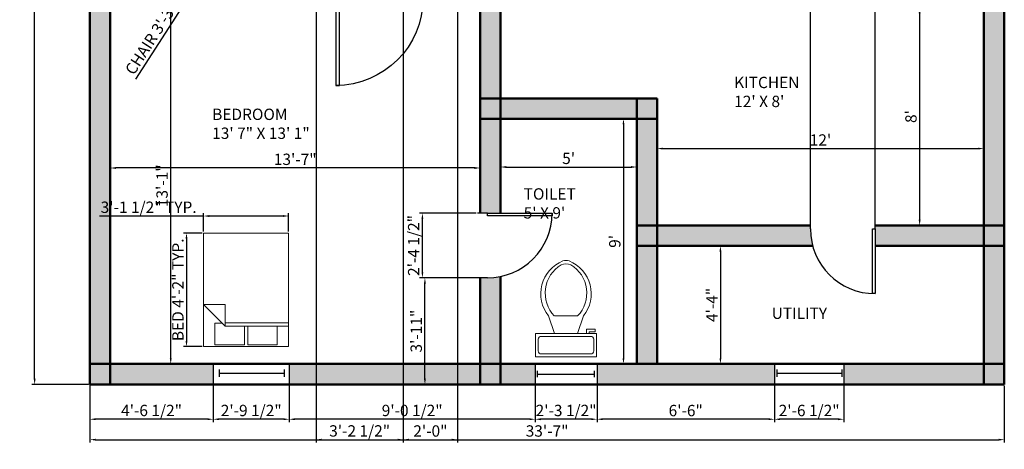
# Model space of a CAD drawing. Units: millimetres. Extents: x 3012 to 3478, y 929 to 1463.
# Tile 1 of 4: x 3012 to 3446, y 929 to 1118. Entities that reach past the tile are written whole.
import ezdxf

# ---------------------------------------------------------------- set-up
doc = ezdxf.new("R2010")
doc.units = ezdxf.units.MM
for name, color, linetype, lineweight in [('A-ANNO-DIMS', 50, 'Continuous', 18), ('A-AREA-IDEN', 170, 'Continuous', 25), ('A-FLOR-FIXT', 9, 'Continuous', 18), ('A-WALL-PATT', 252, 'Continuous', 13), ('doors', 130, 'Continuous', 25), ('furniture', 80, 'Continuous', 18), ('walls', 10, 'Continuous', 50), ('windows', 40, 'Continuous', 25)]:
    doc.layers.add(name, color=color, linetype=linetype, lineweight=lineweight)
doc.styles.get("Standard").update_dxf_attribs({"font": 'arial.ttf'})
doc.dimstyles.new('ISO-25', dxfattribs={"dimtxt": 5, "dimasz": 2.5, "dimexe": 1.25, "dimexo": 0.625, "dimtad": 1, "dimdec": 0, "dimlunit": 3, "dimtxsty": 'Standard', "dimcen": 2.5, "dimadec": 0, "dimazin": 0, "dimtfac": 1, "dimtdec": 0, "dimtmove": 0, "dimatfit": 3, "dimfxl": 1, "dimarcsym": 0})

# ---------------------------------------------------------------- blocks, each defined once
blk = doc.blocks.new('*U2')
for p, q in [((0, 0), (0, -6)), ((40, 0), (40, -6))]:
    blk.add_line(p, q)
blk.add_lwpolyline([(0, 0), (0, 40), (1.75, 40), (1.75, 0)], close=True)
blk.add_arc((0, 0), 40, 0, 90)
blk = doc.blocks.new('*U4')
for p, q in [((0, 4), (0, 0)), ((0, 2), (36, 2)), ((36, 4), (36, 0))]:
    blk.add_line(p, q)
blk = doc.blocks.new('*U5')
for p, q in [((0, 4), (0, 0)), ((0, 2), (36, 2)), ((36, 4), (36, 0))]:
    blk.add_line(p, q)
blk = doc.blocks.new('Bed - Queen')
for p, q in [((0, -80.00003), (0, 0)), ((0, 0), (59.99999, 0)), ((59.99999, 0), (59.99999, -80.00003)), ((7.99999, -1.2), (28.79998, -1.2)), ((7.99999, -14.4), (7.99999, -1.2)), ((28.79998, -1.2), (28.79998, -14.4)), ((31.19999, -1.2), (51.99999, -1.2)), ((31.19999, -14.4), (31.19999, -1.2)), ((51.99999, -1.2), (51.99999, -16.4)), ((0, -14.4), (44.8, -14.4)), ((44.8, -16.8), (0, -16.8)), ((59.99999, -29.6), (44.8, -14.4)), ((44.8, -14.4), (44.8, -29.6)), ((51.99999, -16.4), (46.79936, -16.4)), ((44.8, -29.6), (59.99999, -29.6)), ((59.99999, -80.00003), (0, -80.00003))]:
    blk.add_line(p, q)
blk = doc.blocks.new('Toilet - top')
for p, q in [((9.5, -6), (9.5, -2)), ((-10, -8.5), (-8, -8.5)), ((-10, -9.5), (-10, -8.5)), ((-7, -9.5), (-10, -9.5)), ((-8, -8.5), (-8, -8)), ((-7, -8), (-7, -9.5)), ((-4, -8), (-6, -14)), ((4, -8), (6, -14)), ((4, -14), (-4, -14))]:
    blk.add_line(p, q)
blk.add_lwpolyline([(10.5, -8), (10.5, 0), (-10.5, 0), (-10.5, -8)], close=True)
for points in [[(-9.5, -2), (-9.5, -6)], [(8.5, -1), (-8.5, -1)], [(-8.5, -7), (8.5, -7)]]:
    blk.add_lwpolyline(points)
for centre, radius, start, end in [((-8.62, -1.88), 0.884, 81.8699, 188.1301), ((8.62, -1.88), 0.884, 351.8699, 98.1301), ((-8.62, -6.12), 0.884, 171.8699, 278.1301), ((8.62, -6.12), 0.884, 261.8699, 8.1301), ((3.52, -21.58), 12.17, 141.4691, 247.9714), ((4.2, -21.82), 11.33, 136.3677, 238.9468), ((-3.52, -21.58), 12.17, 292.0284, 38.5307), ((-4.2, -21.82), 11.33, 301.053, 43.6321), ((0, -27.88), 4, 245.7318, 294.2682), ((0, -29), 4, 254.8605, 285.1395)]:
    blk.add_arc(centre, radius, start, end)
blk = doc.blocks.new('*D18')
at = {"layer": 'A-ANNO-DIMS', "color": 0, "lineweight": -2, "transparency": 16777216}
for p, q in [((3052.21, 1061.74), (3052.21, 1051.52)), ((3215.21, 1061.74), (3215.21, 1051.52)), ((3212.71, 1052.77), (3054.71, 1052.77))]:
    blk.add_line(p, q, dxfattribs=at)
at = {"layer": 'A-ANNO-DIMS', "color": 0, "transparency": 16777216}
for points in [[(3054.71, 1053.19), (3054.71, 1052.35), (3052.21, 1052.77)], [(3212.71, 1053.19), (3212.71, 1052.35), (3215.21, 1052.77)]]:
    blk.add_solid(points, dxfattribs=at)
at = {"layer": 'Defpoints', "color": 0, "transparency": 16777216}
for p in [(3052.21, 1062.37), (3215.21, 1062.37), (3052.21, 1052.77)]:
    blk.add_point(p, dxfattribs=at)
at = {"layer": 'A-ANNO-DIMS', "color": 0, "transparency": 16777216, "insert": (3133.71, 1055.95), "char_height": 5, "attachment_point": 5}
blk.add_mtext('13\'-7"', dxfattribs=at)
blk = doc.blocks.new('*D19')
at = {"layer": 'A-ANNO-DIMS', "color": 0, "lineweight": -2, "transparency": 16777216}
for p, q in [((3065.42, 1123.44), (3080.09, 1123.44)), ((3078.84, 968.94), (3078.84, 1120.94)), ((3065.42, 966.44), (3080.09, 966.44))]:
    blk.add_line(p, q, dxfattribs=at)
at = {"layer": 'A-ANNO-DIMS', "color": 0, "transparency": 16777216}
for points in [[(3078.43, 1120.94), (3079.26, 1120.94), (3078.84, 1123.44)], [(3078.43, 968.94), (3079.26, 968.94), (3078.84, 966.44)]]:
    blk.add_solid(points, dxfattribs=at)
at = {"layer": 'Defpoints', "color": 0, "transparency": 16777216}
for p in [(3064.8, 1123.44), (3078.84, 1123.44), (3064.8, 966.44)]:
    blk.add_point(p, dxfattribs=at)
at = {"layer": 'A-ANNO-DIMS', "color": 0, "transparency": 16777216, "insert": (3075.66, 1044.94), "char_height": 5, "attachment_point": 5, "rotation": 90}
blk.add_mtext('13\'-1"', dxfattribs=at)
blk = doc.blocks.new('*D20')
at = {"layer": 'A-ANNO-DIMS', "color": 0, "lineweight": -2, "transparency": 16777216}
for p, q in [((3277.29, 1074.44), (3279.62, 1074.44)), ((3278.37, 1071.94), (3278.37, 968.94)), ((3277.29, 966.44), (3279.62, 966.44))]:
    blk.add_line(p, q, dxfattribs=at)
at = {"layer": 'A-ANNO-DIMS', "color": 0, "transparency": 16777216}
for points in [[(3277.96, 1071.94), (3278.79, 1071.94), (3278.37, 1074.44)], [(3277.96, 968.94), (3278.79, 968.94), (3278.37, 966.44)]]:
    blk.add_solid(points, dxfattribs=at)
at = {"layer": 'Defpoints', "color": 0, "transparency": 16777216}
for p in [(3276.67, 1074.44), (3276.67, 966.44), (3278.37, 966.44)]:
    blk.add_point(p, dxfattribs=at)
at = {"layer": 'A-ANNO-DIMS', "color": 0, "transparency": 16777216, "insert": (3275.2, 1020.44), "char_height": 5, "attachment_point": 5, "rotation": 90}
blk.add_mtext("9'", dxfattribs=at)
blk = doc.blocks.new('*D21')
at = {"layer": 'A-ANNO-DIMS', "color": 0, "lineweight": -2, "transparency": 16777216}
for p, q in [((3224.21, 1053.83), (3224.21, 1054.45)), ((3226.71, 1053.2), (3281.71, 1053.2)), ((3284.21, 1053.83), (3284.21, 1054.45))]:
    blk.add_line(p, q, dxfattribs=at)
at = {"layer": 'A-ANNO-DIMS', "color": 0, "transparency": 16777216}
for points in [[(3226.71, 1053.62), (3226.71, 1052.78), (3224.21, 1053.2)], [(3281.71, 1053.62), (3281.71, 1052.78), (3284.21, 1053.2)]]:
    blk.add_solid(points, dxfattribs=at)
at = {"layer": 'Defpoints', "color": 0, "transparency": 16777216}
for p in [(3224.21, 1053.2), (3284.21, 1053.2), (3284.21, 1053.2)]:
    blk.add_point(p, dxfattribs=at)
at = {"layer": 'A-ANNO-DIMS', "color": 0, "transparency": 16777216, "insert": (3254.21, 1056.37), "char_height": 5, "attachment_point": 5}
blk.add_mtext("5'", dxfattribs=at)
blk = doc.blocks.new('*D22')
at = {"layer": 'A-ANNO-DIMS', "color": 0, "lineweight": -2, "transparency": 16777216}
for p, q in [((3322.37, 1018.44), (3319.85, 1018.44)), ((3321.1, 1015.94), (3321.1, 968.94)), ((3322.37, 966.44), (3319.85, 966.44))]:
    blk.add_line(p, q, dxfattribs=at)
at = {"layer": 'A-ANNO-DIMS', "color": 0, "transparency": 16777216}
for points in [[(3320.68, 1015.94), (3321.51, 1015.94), (3321.1, 1018.44)], [(3320.68, 968.94), (3321.51, 968.94), (3321.1, 966.44)]]:
    blk.add_solid(points, dxfattribs=at)
at = {"layer": 'Defpoints', "color": 0, "transparency": 16777216}
for p in [(3322.99, 1018.44), (3321.1, 966.44), (3322.99, 966.44)]:
    blk.add_point(p, dxfattribs=at)
at = {"layer": 'A-ANNO-DIMS', "color": 0, "transparency": 16777216, "insert": (3317.97, 992.44), "char_height": 5, "attachment_point": 5, "rotation": 90}
blk.add_mtext('4\'-4"', dxfattribs=at)
blk = doc.blocks.new('*D23')
at = {"layer": 'A-ANNO-DIMS', "color": 0, "lineweight": -2, "transparency": 16777216}
for p, q in [((3408.9, 1120.94), (3408.9, 1029.94)), ((3409.52, 1123.44), (3410.15, 1123.44)), ((3409.52, 1027.44), (3410.15, 1027.44))]:
    blk.add_line(p, q, dxfattribs=at)
at = {"layer": 'A-ANNO-DIMS', "color": 0, "transparency": 16777216}
for points in [[(3408.48, 1120.94), (3409.31, 1120.94), (3408.9, 1123.44)], [(3408.48, 1029.94), (3409.31, 1029.94), (3408.9, 1027.44)]]:
    blk.add_solid(points, dxfattribs=at)
at = {"layer": 'Defpoints', "color": 0, "transparency": 16777216}
for p in [(3408.9, 1123.44), (3408.9, 1027.44), (3408.9, 1027.44)]:
    blk.add_point(p, dxfattribs=at)
at = {"layer": 'A-ANNO-DIMS', "color": 0, "transparency": 16777216, "insert": (3405.72, 1075.44), "char_height": 5, "attachment_point": 5, "rotation": 90}
blk.add_mtext("8'", dxfattribs=at)
blk = doc.blocks.new('*D24')
at = {"layer": 'A-ANNO-DIMS', "color": 0, "lineweight": -2, "transparency": 16777216}
for p, q in [((3293.21, 1055.32), (3293.21, 1062.57)), ((3295.71, 1061.32), (3434.71, 1061.32)), ((3437.21, 1055.32), (3437.21, 1062.57))]:
    blk.add_line(p, q, dxfattribs=at)
at = {"layer": 'A-ANNO-DIMS', "color": 0, "transparency": 16777216}
for points in [[(3295.71, 1061.74), (3295.71, 1060.91), (3293.21, 1061.32)], [(3434.71, 1061.74), (3434.71, 1060.91), (3437.21, 1061.32)]]:
    blk.add_solid(points, dxfattribs=at)
at = {"layer": 'Defpoints', "color": 0, "transparency": 16777216}
for p in [(3437.21, 1061.32), (3293.21, 1054.7), (3437.21, 1054.7)]:
    blk.add_point(p, dxfattribs=at)
at = {"layer": 'A-ANNO-DIMS', "color": 0, "transparency": 16777216, "insert": (3365.21, 1064.46), "char_height": 5, "attachment_point": 5}
blk.add_mtext("12'", dxfattribs=at)
blk = doc.blocks.new('*D30')
at = {"layer": 'A-ANNO-DIMS', "color": 0, "lineweight": -2, "transparency": 16777216}
for p, q in [((3092.67, 1024.12), (3084.54, 1024.12)), ((3085.79, 1021.62), (3085.79, 976.61)), ((3092.67, 974.11), (3084.54, 974.11))]:
    blk.add_line(p, q, dxfattribs=at)
at = {"layer": 'A-ANNO-DIMS', "color": 0, "transparency": 16777216}
for points in [[(3085.38, 1021.62), (3086.21, 1021.62), (3085.79, 1024.12)], [(3085.38, 976.61), (3086.21, 976.61), (3085.79, 974.11)]]:
    blk.add_solid(points, dxfattribs=at)
at = {"layer": 'Defpoints', "color": 0, "transparency": 16777216}
for p in [(3093.3, 1024.12), (3085.79, 974.11), (3093.3, 974.11)]:
    blk.add_point(p, dxfattribs=at)
at = {"layer": 'A-ANNO-DIMS', "color": 0, "transparency": 16777216, "insert": (3082.66, 999.11), "char_height": 5, "attachment_point": 5, "rotation": 90}
blk.add_mtext('BED 4\'-2" TYP.', dxfattribs=at)
blk = doc.blocks.new('*D31')
at = {"layer": 'A-ANNO-DIMS', "color": 0, "lineweight": -2, "transparency": 16777216}
for p, q in [((3093.3, 1024.74), (3093.3, 1032.87)), ((3130.81, 1024.74), (3130.81, 1032.87)), ((3093.3, 1031.62), (3047.42, 1031.62)), ((3128.31, 1031.62), (3095.8, 1031.62))]:
    blk.add_line(p, q, dxfattribs=at)
at = {"layer": 'A-ANNO-DIMS', "color": 0, "transparency": 16777216}
for points in [[(3095.8, 1032.04), (3095.8, 1031.2), (3093.3, 1031.62)], [(3128.31, 1032.04), (3128.31, 1031.2), (3130.81, 1031.62)]]:
    blk.add_solid(points, dxfattribs=at)
at = {"layer": 'Defpoints', "color": 0, "transparency": 16777216}
for p in [(3093.3, 1031.62), (3093.3, 1024.12), (3130.81, 1024.12)]:
    blk.add_point(p, dxfattribs=at)
at = {"layer": 'A-ANNO-DIMS', "color": 0, "transparency": 16777216, "insert": (3069.11, 1034.83), "char_height": 5, "attachment_point": 5}
blk.add_mtext('3\'-1 1/2" TYP.', dxfattribs=at)
blk = doc.blocks.new('*D40')
at = {"layer": 'A-ANNO-DIMS', "color": 0, "lineweight": -2, "transparency": 16777216}
for p, q in [((3108.55, 1171.79), (3114.04, 1168.25)), ((3111.63, 1166.83), (3093, 1137.95)), ((3087.21, 1138.72), (3092.7, 1135.18)), ((3091.65, 1135.85), (3063.29, 1091.9))]:
    blk.add_line(p, q, dxfattribs=at)
at = {"layer": 'A-ANNO-DIMS', "color": 0, "transparency": 16777216}
for points in [[(3111.28, 1167.05), (3111.98, 1166.6), (3112.99, 1168.93)], [(3092.65, 1138.18), (3093.35, 1137.73), (3091.65, 1135.85)]]:
    blk.add_solid(points, dxfattribs=at)
at = {"layer": 'Defpoints', "color": 0, "transparency": 16777216}
for p in [(3108.03, 1172.13), (3086.69, 1139.06), (3091.65, 1135.85)]:
    blk.add_point(p, dxfattribs=at)
at = {"layer": 'A-ANNO-DIMS', "color": 0, "transparency": 16777216, "insert": (3074.09, 1114.57), "char_height": 5, "attachment_point": 5, "rotation": 57.1659}
blk.add_mtext('CHAIR 3\'-3 1/2"', dxfattribs=at)
blk = doc.blocks.new('*D42')
at = {"layer": 'A-ANNO-DIMS', "color": 0, "lineweight": -2, "transparency": 16777216}
for p, q in [((3042.59, 1414.44), (3017.61, 1414.44)), ((3018.86, 959.94), (3018.86, 1411.94)), ((3042.59, 957.44), (3017.61, 957.44))]:
    blk.add_line(p, q, dxfattribs=at)
at = {"layer": 'A-ANNO-DIMS', "color": 0, "transparency": 16777216}
for points in [[(3018.45, 1411.94), (3019.28, 1411.94), (3018.86, 1414.44)], [(3018.45, 959.94), (3019.28, 959.94), (3018.86, 957.44)]]:
    blk.add_solid(points, dxfattribs=at)
at = {"layer": 'Defpoints', "color": 0, "transparency": 16777216}
for p in [(3018.86, 1414.44), (3043.21, 1414.44), (3043.21, 957.44)]:
    blk.add_point(p, dxfattribs=at)
at = {"layer": 'A-ANNO-DIMS', "color": 0, "transparency": 16777216, "insert": (3015.68, 1185.94), "char_height": 5, "attachment_point": 5, "rotation": 90}
blk.add_mtext('38\'-1"', dxfattribs=at)
blk = doc.blocks.new('*D49')
at = {"layer": 'A-ANNO-DIMS', "color": 0, "lineweight": -2, "transparency": 16777216}
for p, q in [((3043.21, 965.82), (3043.21, 940.84)), ((3097.57, 965.82), (3097.57, 940.84)), ((3095.07, 942.09), (3045.71, 942.09))]:
    blk.add_line(p, q, dxfattribs=at)
at = {"layer": 'A-ANNO-DIMS', "color": 0, "transparency": 16777216}
for points in [[(3045.71, 942.51), (3045.71, 941.68), (3043.21, 942.09)], [(3095.07, 942.51), (3095.07, 941.68), (3097.57, 942.09)]]:
    blk.add_solid(points, dxfattribs=at)
at = {"layer": 'Defpoints', "color": 0, "transparency": 16777216}
for p in [(3043.21, 966.44), (3097.57, 966.44), (3043.21, 942.09)]:
    blk.add_point(p, dxfattribs=at)
at = {"layer": 'A-ANNO-DIMS', "color": 0, "transparency": 16777216, "insert": (3070.39, 945.3), "char_height": 5, "attachment_point": 5}
blk.add_mtext('4\'-6 1/2"', dxfattribs=at)
blk = doc.blocks.new('*D50')
at = {"layer": 'A-ANNO-DIMS', "color": 0, "lineweight": -2, "transparency": 16777216}
for p, q in [((3097.57, 965.82), (3097.57, 940.84)), ((3131.05, 965.82), (3131.05, 940.84)), ((3128.55, 942.09), (3100.07, 942.09))]:
    blk.add_line(p, q, dxfattribs=at)
at = {"layer": 'A-ANNO-DIMS', "color": 0, "transparency": 16777216}
for points in [[(3100.07, 942.51), (3100.07, 941.68), (3097.57, 942.09)], [(3128.55, 942.51), (3128.55, 941.68), (3131.05, 942.09)]]:
    blk.add_solid(points, dxfattribs=at)
at = {"layer": 'Defpoints', "color": 0, "transparency": 16777216}
for p in [(3097.57, 966.44), (3131.05, 966.44), (3097.57, 942.09)]:
    blk.add_point(p, dxfattribs=at)
at = {"layer": 'A-ANNO-DIMS', "color": 0, "transparency": 16777216, "insert": (3114.31, 945.3), "char_height": 5, "attachment_point": 5}
blk.add_mtext('2\'-9 1/2"', dxfattribs=at)
blk = doc.blocks.new('*D51')
at = {"layer": 'A-ANNO-DIMS', "color": 0, "lineweight": -2, "transparency": 16777216}
for p, q in [((3131.05, 965.82), (3131.05, 940.84)), ((3239.46, 965.82), (3239.46, 940.84)), ((3236.96, 942.09), (3133.55, 942.09))]:
    blk.add_line(p, q, dxfattribs=at)
at = {"layer": 'A-ANNO-DIMS', "color": 0, "transparency": 16777216}
for points in [[(3133.55, 942.51), (3133.55, 941.68), (3131.05, 942.09)], [(3236.96, 942.51), (3236.96, 941.68), (3239.46, 942.09)]]:
    blk.add_solid(points, dxfattribs=at)
at = {"layer": 'Defpoints', "color": 0, "transparency": 16777216}
for p in [(3131.05, 966.44), (3239.46, 966.44), (3131.05, 942.09)]:
    blk.add_point(p, dxfattribs=at)
at = {"layer": 'A-ANNO-DIMS', "color": 0, "transparency": 16777216, "insert": (3185.25, 945.3), "char_height": 5, "attachment_point": 5}
blk.add_mtext('9\'-0 1/2"', dxfattribs=at)
blk = doc.blocks.new('*D52')
at = {"layer": 'A-ANNO-DIMS', "color": 0, "lineweight": -2, "transparency": 16777216}
for p, q in [((3239.46, 965.82), (3239.46, 940.84)), ((3266.71, 965.82), (3266.71, 940.84)), ((3264.21, 942.09), (3241.96, 942.09))]:
    blk.add_line(p, q, dxfattribs=at)
at = {"layer": 'A-ANNO-DIMS', "color": 0, "transparency": 16777216}
for points in [[(3241.96, 942.51), (3241.96, 941.68), (3239.46, 942.09)], [(3264.21, 942.51), (3264.21, 941.68), (3266.71, 942.09)]]:
    blk.add_solid(points, dxfattribs=at)
at = {"layer": 'Defpoints', "color": 0, "transparency": 16777216}
for p in [(3239.46, 966.44), (3266.71, 966.44), (3239.46, 942.09)]:
    blk.add_point(p, dxfattribs=at)
at = {"layer": 'A-ANNO-DIMS', "color": 0, "transparency": 16777216, "insert": (3253.08, 945.3), "char_height": 5, "attachment_point": 5}
blk.add_mtext('2\'-3 1/2"', dxfattribs=at)
blk = doc.blocks.new('*D53')
at = {"layer": 'A-ANNO-DIMS', "color": 0, "lineweight": -2, "transparency": 16777216}
for p, q in [((3266.71, 965.82), (3266.71, 940.84)), ((3344.91, 965.82), (3344.91, 940.84)), ((3342.41, 942.09), (3269.21, 942.09))]:
    blk.add_line(p, q, dxfattribs=at)
at = {"layer": 'A-ANNO-DIMS', "color": 0, "transparency": 16777216}
for points in [[(3269.21, 942.51), (3269.21, 941.68), (3266.71, 942.09)], [(3342.41, 942.51), (3342.41, 941.68), (3344.91, 942.09)]]:
    blk.add_solid(points, dxfattribs=at)
at = {"layer": 'Defpoints', "color": 0, "transparency": 16777216}
for p in [(3266.71, 966.44), (3344.91, 966.44), (3266.71, 942.09)]:
    blk.add_point(p, dxfattribs=at)
at = {"layer": 'A-ANNO-DIMS', "color": 0, "transparency": 16777216, "insert": (3305.81, 945.27), "char_height": 5, "attachment_point": 5}
blk.add_mtext('6\'-6"', dxfattribs=at)
blk = doc.blocks.new('*D54')
at = {"layer": 'A-ANNO-DIMS', "color": 0, "lineweight": -2, "transparency": 16777216}
for p, q in [((3344.91, 965.82), (3344.91, 940.84)), ((3375.49, 965.82), (3375.49, 940.84)), ((3372.99, 942.09), (3347.41, 942.09))]:
    blk.add_line(p, q, dxfattribs=at)
at = {"layer": 'A-ANNO-DIMS', "color": 0, "transparency": 16777216}
for points in [[(3347.41, 942.51), (3347.41, 941.68), (3344.91, 942.09)], [(3372.99, 942.51), (3372.99, 941.68), (3375.49, 942.09)]]:
    blk.add_solid(points, dxfattribs=at)
at = {"layer": 'Defpoints', "color": 0, "transparency": 16777216}
for p in [(3344.91, 966.44), (3375.49, 966.44), (3344.91, 942.09)]:
    blk.add_point(p, dxfattribs=at)
at = {"layer": 'A-ANNO-DIMS', "color": 0, "transparency": 16777216, "insert": (3360.2, 945.3), "char_height": 5, "attachment_point": 5}
blk.add_mtext('2\'-6 1/2"', dxfattribs=at)
blk = doc.blocks.new('*D57')
at = {"layer": 'A-ANNO-DIMS', "color": 0, "lineweight": -2, "transparency": 16777216}
for p, q in [((3142.87, 1263.82), (3142.87, 931.84)), ((3181.32, 1263.82), (3181.32, 931.84)), ((3145.37, 933.09), (3178.82, 933.09))]:
    blk.add_line(p, q, dxfattribs=at)
at = {"layer": 'A-ANNO-DIMS', "color": 0, "transparency": 16777216}
for points in [[(3145.37, 933.51), (3145.37, 932.68), (3142.87, 933.09)], [(3178.82, 933.51), (3178.82, 932.68), (3181.32, 933.09)]]:
    blk.add_solid(points, dxfattribs=at)
at = {"layer": 'Defpoints', "color": 0, "transparency": 16777216}
for p in [(3142.87, 1264.44), (3181.32, 1264.44), (3181.32, 933.09)]:
    blk.add_point(p, dxfattribs=at)
at = {"layer": 'A-ANNO-DIMS', "color": 0, "transparency": 16777216, "insert": (3162.1, 936.3), "char_height": 5, "attachment_point": 5}
blk.add_mtext('3\'-2 1/2"', dxfattribs=at)
blk = doc.blocks.new('*D58')
at = {"layer": 'A-ANNO-DIMS', "color": 0, "lineweight": -2, "transparency": 16777216}
for p, q in [((3181.32, 1263.82), (3181.32, 931.84)), ((3205.21, 1263.82), (3205.21, 931.84)), ((3183.82, 933.09), (3202.71, 933.09))]:
    blk.add_line(p, q, dxfattribs=at)
at = {"layer": 'A-ANNO-DIMS', "color": 0, "transparency": 16777216}
for points in [[(3183.82, 933.51), (3183.82, 932.68), (3181.32, 933.09)], [(3202.71, 933.51), (3202.71, 932.68), (3205.21, 933.09)]]:
    blk.add_solid(points, dxfattribs=at)
at = {"layer": 'Defpoints', "color": 0, "transparency": 16777216}
for p in [(3181.32, 1264.44), (3205.21, 1264.44), (3205.21, 933.09)]:
    blk.add_point(p, dxfattribs=at)
at = {"layer": 'A-ANNO-DIMS', "color": 0, "transparency": 16777216, "insert": (3193.27, 936.27), "char_height": 5, "attachment_point": 5}
blk.add_mtext('2\'-0"', dxfattribs=at)
blk = doc.blocks.new('*D63')
at = {"layer": 'A-ANNO-DIMS', "color": 0, "lineweight": -2, "transparency": 16777216}
for p, q in [((3213.49, 1032.91), (3188.51, 1032.91)), ((3189.76, 1006.87), (3189.76, 1030.41)), ((3213.49, 1004.37), (3188.51, 1004.37))]:
    blk.add_line(p, q, dxfattribs=at)
at = {"layer": 'A-ANNO-DIMS', "color": 0, "transparency": 16777216}
for points in [[(3189.34, 1030.41), (3190.18, 1030.41), (3189.76, 1032.91)], [(3189.34, 1006.87), (3190.18, 1006.87), (3189.76, 1004.37)]]:
    blk.add_solid(points, dxfattribs=at)
at = {"layer": 'Defpoints', "color": 0, "transparency": 16777216}
for p in [(3189.76, 1032.91), (3214.11, 1032.91), (3214.11, 1004.37)]:
    blk.add_point(p, dxfattribs=at)
at = {"layer": 'A-ANNO-DIMS', "color": 0, "transparency": 16777216, "insert": (3186.55, 1018.64), "char_height": 5, "attachment_point": 5, "rotation": 90}
blk.add_mtext('2\'-4 1/2"', dxfattribs=at)
blk = doc.blocks.new('*D64')
at = {"layer": 'A-ANNO-DIMS', "color": 0, "lineweight": -2, "transparency": 16777216}
for p, q in [((3214.59, 1004.37), (3189.61, 1004.37)), ((3190.86, 959.94), (3190.86, 1001.87)), ((3214.59, 957.44), (3189.61, 957.44))]:
    blk.add_line(p, q, dxfattribs=at)
at = {"layer": 'A-ANNO-DIMS', "color": 0, "transparency": 16777216}
for points in [[(3190.45, 1001.87), (3191.28, 1001.87), (3190.86, 1004.37)], [(3190.45, 959.94), (3191.28, 959.94), (3190.86, 957.44)]]:
    blk.add_solid(points, dxfattribs=at)
at = {"layer": 'Defpoints', "color": 0, "transparency": 16777216}
for p in [(3190.86, 1004.37), (3215.21, 1004.37), (3215.21, 957.44)]:
    blk.add_point(p, dxfattribs=at)
at = {"layer": 'A-ANNO-DIMS', "color": 0, "transparency": 16777216, "insert": (3187.68, 980.91), "char_height": 5, "attachment_point": 5, "rotation": 90}
blk.add_mtext('3\'-11"', dxfattribs=at)
blk = doc.blocks.new('*D65')
at = {"layer": 'A-ANNO-DIMS', "color": 0, "lineweight": -2, "transparency": 16777216}
for p, q in [((3360.77, 1028.07), (3360.77, 1440.04)), ((3363.27, 1438.79), (3386.8, 1438.79)), ((3389.3, 1028.07), (3389.3, 1440.04))]:
    blk.add_line(p, q, dxfattribs=at)
at = {"layer": 'A-ANNO-DIMS', "color": 0, "transparency": 16777216}
for points in [[(3363.27, 1439.21), (3363.27, 1438.38), (3360.77, 1438.79)], [(3386.8, 1439.21), (3386.8, 1438.38), (3389.3, 1438.79)]]:
    blk.add_solid(points, dxfattribs=at)
at = {"layer": 'Defpoints', "color": 0, "transparency": 16777216}
for p in [(3389.3, 1438.79), (3360.77, 1027.44), (3389.3, 1027.44)]:
    blk.add_point(p, dxfattribs=at)
at = {"layer": 'A-ANNO-DIMS', "color": 0, "transparency": 16777216, "insert": (3375.03, 1442), "char_height": 5, "attachment_point": 5}
blk.add_mtext('2\'-4 1/2"', dxfattribs=at)
blk = doc.blocks.new('*D66')
at = {"layer": 'A-ANNO-DIMS', "color": 0, "lineweight": -2, "transparency": 16777216}
for p, q in [((3389.3, 1028.07), (3389.3, 1440.04)), ((3391.8, 1438.79), (3443.71, 1438.79)), ((3446.21, 1028.07), (3446.21, 1440.04))]:
    blk.add_line(p, q, dxfattribs=at)
at = {"layer": 'A-ANNO-DIMS', "color": 0, "transparency": 16777216}
for points in [[(3391.8, 1439.21), (3391.8, 1438.38), (3389.3, 1438.79)], [(3443.71, 1439.21), (3443.71, 1438.38), (3446.21, 1438.79)]]:
    blk.add_solid(points, dxfattribs=at)
at = {"layer": 'Defpoints', "color": 0, "transparency": 16777216}
for p in [(3446.21, 1438.79), (3389.3, 1027.44), (3446.21, 1027.44)]:
    blk.add_point(p, dxfattribs=at)
at = {"layer": 'A-ANNO-DIMS', "color": 0, "transparency": 16777216, "insert": (3417.76, 1441.97), "char_height": 5, "attachment_point": 5}
blk.add_mtext('4\'-9"', dxfattribs=at)
blk = doc.blocks.new('*D74')
at = {"layer": 'A-ANNO-DIMS', "color": 0, "lineweight": -2, "transparency": 16777216}
for p, q in [((3043.21, 956.82), (3043.21, 931.84)), ((3446.21, 956.82), (3446.21, 931.84)), ((3045.71, 933.09), (3443.71, 933.09))]:
    blk.add_line(p, q, dxfattribs=at)
at = {"layer": 'A-ANNO-DIMS', "color": 0, "transparency": 16777216}
for points in [[(3045.71, 933.51), (3045.71, 932.68), (3043.21, 933.09)], [(3443.71, 933.51), (3443.71, 932.68), (3446.21, 933.09)]]:
    blk.add_solid(points, dxfattribs=at)
at = {"layer": 'Defpoints', "color": 0, "transparency": 16777216}
for p in [(3043.21, 957.44), (3446.21, 957.44), (3446.21, 933.09)]:
    blk.add_point(p, dxfattribs=at)
at = {"layer": 'A-ANNO-DIMS', "color": 0, "transparency": 16777216, "insert": (3244.71, 936.27), "char_height": 5, "attachment_point": 5}
blk.add_mtext('33\'-7"', dxfattribs=at)

msp = doc.modelspace()

# ---------------------------------------------------------------- hatches: boundary and pattern name
at = {"layer": 'A-WALL-PATT'}
h = msp.add_hatch(color=256, dxfattribs=at)
h.dxf.hatch_style = 1
h.paths.add_polyline_path([(3052.21, 1405.44), (3043.21, 1405.44), (3043.21, 1273.44), (3052.21, 1273.44)])
h.paths.add_polyline_path([(3052.21, 1273.44), (3043.21, 1273.44), (3043.21, 1264.44), (3052.21, 1264.44)])
h.paths.add_polyline_path([(3052.21, 1264.44), (3043.21, 1264.44), (3043.21, 1132.44), (3052.21, 1132.44)])
h.paths.add_polyline_path([(3116.21, 1273.44), (3052.21, 1273.44), (3052.21, 1264.44), (3116.21, 1264.44)])
h.paths.add_polyline_path([(3125.21, 1273.44), (3116.21, 1273.44), (3116.21, 1264.44), (3125.21, 1264.44)])
h.paths.add_polyline_path([(3143.26, 1273.44), (3125.21, 1273.44), (3125.21, 1264.44), (3142.87, 1264.44), (3142.87, 1268, -0.035543)])
h.paths.add_polyline_path([(3052.21, 1414.44), (3043.21, 1414.44), (3043.21, 1405.44), (3052.21, 1405.44)])
h.paths.add_polyline_path([(3096.89, 1414.44), (3052.21, 1414.44), (3052.21, 1405.44), (3096.89, 1405.44)])
h.paths.add_polyline_path([(3196.21, 1414.44), (3129.12, 1414.44), (3129.12, 1405.44), (3196.21, 1405.44)])
h.paths.add_polyline_path([(3205.21, 1414.44), (3196.21, 1414.44), (3196.21, 1405.44), (3205.21, 1405.44)])
h.paths.add_polyline_path([(3205.21, 1405.44), (3196.21, 1405.44), (3196.21, 1321.44), (3205.21, 1321.44)])
h.paths.add_polyline_path([(3205.21, 1321.44), (3196.21, 1321.44), (3196.21, 1312.44), (3205.21, 1312.44)])
h.paths.add_polyline_path([(3205.21, 1312.44), (3196.21, 1312.44), (3196.21, 1273.44), (3205.21, 1273.44)])
h.paths.add_polyline_path([(3284.21, 1321.44), (3205.21, 1321.44), (3205.21, 1312.44), (3284.21, 1312.44)])
h.paths.add_polyline_path([(3205.21, 1273.44), (3196.21, 1273.44), (3196.21, 1264.44), (3205.21, 1264.44)])
h.paths.add_polyline_path([(3196.21, 1273.44), (3181.32, 1273.44), (3181.32, 1268), (3181.32, 1264.44), (3196.21, 1264.44)])
h.paths.add_polyline_path([(3293.21, 1405.44), (3284.21, 1405.44), (3284.21, 1321.44), (3293.21, 1321.44)])
h.paths.add_polyline_path([(3293.21, 1414.44), (3284.21, 1414.44), (3284.21, 1405.44), (3293.21, 1405.44)])
h.paths.add_polyline_path([(3284.21, 1414.44), (3249.55, 1414.44), (3249.55, 1405.44), (3284.21, 1405.44)])
h.paths.add_polyline_path([(3221.79, 1414.44), (3205.21, 1414.44), (3205.21, 1405.44), (3221.79, 1405.44)])
h.paths.add_polyline_path([(3339.87, 1414.44), (3293.21, 1414.44), (3293.21, 1405.44), (3339.87, 1405.44)])
h.paths.add_polyline_path([(3437.21, 1414.44), (3373.17, 1414.44), (3373.17, 1405.44), (3437.21, 1405.44)])
h.paths.add_polyline_path([(3446.21, 1414.44), (3437.21, 1414.44), (3437.21, 1405.44), (3446.21, 1405.44)])
h.paths.add_polyline_path([(3446.21, 1405.44), (3437.21, 1405.44), (3437.21, 1273.44), (3446.21, 1273.44)])
h.paths.add_polyline_path([(3437.21, 1273.44), (3293.21, 1273.44), (3293.21, 1264.44), (3437.21, 1264.44)])
h.paths.add_polyline_path([(3446.21, 1273.44), (3437.21, 1273.44), (3437.21, 1264.44), (3446.21, 1264.44)])
h.paths.add_polyline_path([(3446.21, 1264.44), (3437.21, 1264.44), (3437.21, 1249.83), (3445.52, 1249.83), (3446.21, 1249.83)])
h.paths.add_polyline_path([(3293.21, 1264.44), (3284.21, 1264.44), (3284.21, 1132.44), (3293.21, 1132.44)])
h.paths.add_polyline_path([(3293.21, 1273.44), (3284.21, 1273.44), (3284.21, 1264.44), (3293.21, 1264.44)])
h.paths.add_polyline_path([(3293.21, 1277.22), (3287.47, 1277.22), (3284.21, 1277.22), (3284.21, 1273.44), (3293.21, 1273.44)])
h.paths.add_polyline_path([(3125.21, 1213.86), (3116.21, 1213.86), (3116.21, 1184.42), (3125.21, 1184.42)])
h.paths.add_polyline_path([(3125.21, 1264.44), (3116.21, 1264.44), (3116.21, 1245.36), (3125.21, 1245.36)])
h.paths.add_polyline_path([(3125.21, 1151.51), (3116.21, 1151.51), (3116.21, 1132.44), (3125.21, 1132.44)])
h.paths.add_polyline_path([(3125.21, 1132.44), (3116.21, 1132.44), (3116.21, 1123.44), (3125.21, 1123.44)])
h.paths.add_polyline_path([(3151.56, 1127.56), (3151.56, 1132.44), (3125.21, 1132.44), (3125.21, 1123.44), (3151.56, 1123.44)])
h.paths.add_polyline_path([(3116.21, 1132.44), (3052.21, 1132.44), (3052.21, 1123.44), (3116.21, 1123.44)])
h.paths.add_polyline_path([(3052.21, 1132.44), (3043.21, 1132.44), (3043.21, 1123.44), (3052.21, 1123.44)])
h.paths.add_polyline_path([(3052.21, 1123.44), (3043.21, 1123.44), (3043.21, 966.44), (3052.21, 966.44)])
h.paths.add_polyline_path([(3097.57, 966.44), (3052.21, 966.44), (3052.21, 957.44), (3097.57, 957.44)])
h.paths.add_polyline_path([(3052.21, 966.44), (3043.21, 966.44), (3043.21, 957.44), (3052.21, 957.44)])
h.paths.add_polyline_path([(3215.21, 966.44), (3131.05, 966.44), (3131.05, 957.44), (3215.21, 957.44)])
h.paths.add_polyline_path([(3224.21, 966.44), (3215.21, 966.44), (3215.21, 957.44), (3224.21, 957.44)])
h.paths.add_polyline_path([(3224.21, 1004.97, -0.051409), (3218.39, 1004.37), (3215.21, 1004.37), (3215.21, 966.44), (3224.21, 966.44)])
h.paths.add_polyline_path([(3239.46, 966.44), (3224.21, 966.44), (3224.21, 957.44), (3239.46, 957.44)])
h.paths.add_polyline_path([(3344.91, 966.44), (3266.71, 966.44), (3266.71, 957.44), (3344.91, 957.44)])
h.paths.add_polyline_path([(3293.21, 1018.44), (3284.21, 1018.44), (3284.21, 966.44), (3293.21, 966.44)])
h.paths.add_polyline_path([(3293.21, 1027.44), (3284.21, 1027.44), (3284.21, 1018.44), (3293.21, 1018.44)])
h.paths.add_polyline_path([(3293.21, 1074.44), (3284.21, 1074.44), (3284.21, 1027.44), (3293.21, 1027.44)])
h.paths.add_polyline_path([(3224.21, 1074.44), (3215.21, 1074.44), (3215.21, 1032.91), (3218.39, 1032.91), (3224.21, 1032.91)])
h.paths.add_polyline_path([(3224.21, 1123.44), (3215.21, 1123.44), (3215.21, 1083.44), (3224.21, 1083.44)])
h.paths.add_polyline_path([(3224.21, 1083.44), (3215.21, 1083.44), (3215.21, 1074.44), (3224.21, 1074.44)])
h.paths.add_polyline_path([(3284.21, 1083.44), (3224.21, 1083.44), (3224.21, 1074.44), (3284.21, 1074.44)])
h.paths.add_polyline_path([(3293.21, 1083.44), (3284.21, 1083.44), (3284.21, 1074.44), (3293.21, 1074.44)])
h.paths.add_polyline_path([(3215.21, 1132.44), (3190.01, 1132.44), (3190.01, 1127.56, -0.026825), (3189.79, 1123.44), (3215.21, 1123.44)])
h.paths.add_polyline_path([(3224.21, 1132.44), (3215.21, 1132.44), (3215.21, 1123.44), (3224.21, 1123.44)])
h.paths.add_polyline_path([(3437.21, 1132.44), (3293.21, 1132.44), (3293.21, 1123.44), (3437.21, 1123.44)])
h.paths.add_polyline_path([(3293.21, 1132.44), (3284.21, 1132.44), (3284.21, 1123.44), (3293.21, 1123.44)])
h.paths.add_polyline_path([(3446.21, 1132.44), (3437.21, 1132.44), (3437.21, 1123.44), (3446.21, 1123.44)])
h.paths.add_polyline_path([(3446.21, 1123.44), (3437.21, 1123.44), (3437.21, 1027.44), (3446.21, 1027.44)])
h.paths.add_polyline_path([(3446.21, 1221.29), (3445.52, 1221.29, -0.074007), (3437.21, 1222.53), (3437.21, 1132.44), (3446.21, 1132.44)])
h.paths.add_polyline_path([(3446.21, 1018.44), (3437.21, 1018.44), (3437.21, 966.44), (3446.21, 966.44)])
h.paths.add_polyline_path([(3446.21, 1027.44), (3437.21, 1027.44), (3437.21, 1018.44), (3446.21, 1018.44)])
h.paths.add_polyline_path([(3437.21, 1027.44), (3389.3, 1027.44), (3389.3, 1025.95), (3389.3, 1018.44), (3437.21, 1018.44)])
h.paths.add_polyline_path([(3360.77, 1025.95), (3360.77, 1027.44), (3293.21, 1027.44), (3293.21, 1018.44), (3361.77, 1018.44, -0.066618)])
h.paths.add_polyline_path([(3437.21, 966.44), (3375.49, 966.44), (3375.49, 957.44), (3437.21, 957.44)])
h.paths.add_polyline_path([(3446.21, 966.44), (3437.21, 966.44), (3437.21, 957.44), (3446.21, 957.44)])

# ---------------------------------------------------------------- linework, layer by layer
at = {"layer": 'walls'}
for p, q in [((3043.21, 1414.44), (3043.21, 957.44)), ((3052.21, 1414.44), (3052.21, 957.44)), ((3437.21, 1222.53), (3437.21, 957.44)), ((3446.21, 1221.29), (3446.21, 957.44)), ((3215.21, 1132.44), (3215.21, 1032.91)), ((3224.21, 1132.44), (3224.21, 1032.91)), ((3215.21, 1083.44), (3293.21, 1083.44)), ((3284.21, 1083.44), (3284.21, 966.44)), ((3293.21, 1083.44), (3293.21, 966.44)), ((3215.21, 1074.44), (3293.21, 1074.44)), ((3284.21, 1027.44), (3360.77, 1027.44)), ((3389.3, 1027.44), (3446.21, 1027.44)), ((3284.21, 1018.44), (3361.77, 1018.44)), ((3389.3, 1018.44), (3446.21, 1018.44)), ((3215.21, 1004.37), (3215.21, 957.44)), ((3224.21, 1004.97), (3224.21, 957.44)), ((3043.21, 966.44), (3446.21, 966.44)), ((3043.21, 957.44), (3446.21, 957.44))]:
    msp.add_line(p, q, dxfattribs=at)
at = {"layer": 'windows'}
for p, q in [((3097.57, 966.44), (3097.57, 957.44)), ((3131.05, 966.44), (3131.05, 957.44)), ((3239.46, 966.44), (3239.46, 957.44)), ((3266.71, 966.44), (3266.71, 957.44)), ((3344.91, 966.44), (3344.91, 957.44)), ((3375.49, 966.44), (3375.49, 957.44))]:
    msp.add_line(p, q, dxfattribs=at)

# ---------------------------------------------------------------- block references
at = {"layer": 'A-FLOR-FIXT', "xscale": 1.284488889705511, "yscale": 1.284488889705511, "zscale": 1.284488889705511, "rotation": 180}
msp.add_blockref('Toilet - top', (3253.04, 969.62), dxfattribs=at)
at = {"layer": 'doors'}
for p, xscale, yscale, zscale, rotation in [((3151.56, 1127.56), -0.9611587719732299, 0.9611587719732299, 0.9611587719732299, 180), ((3218.39, 1032.91), 0.7134266761523853, 0.7134266761523853, 0.7134266761523853, 270), ((3389.3, 1025.95), 0.7134266761523853, 0.7134266761523853, 0.7134266761523853, 180)]:
    msp.add_blockref('*U2', p, dxfattribs=dict(at, xscale=xscale, yscale=yscale, zscale=zscale, rotation=rotation))
at = {"layer": 'furniture', "xscale": 0.625172702944318, "yscale": 0.625172702944318, "zscale": 0.625172702944318, "rotation": 180}
msp.add_blockref('Bed - Queen', (3130.81, 974.11), dxfattribs=at)
at = {"layer": 'windows'}
for name, p, xscale, yscale, zscale in [('*U4', (3100.13, 960.83), 0.7972415233030418, 0.7972415233030418, 0.7972415233030418), ('*U5', (3240.38, 960.59), 0.6985876539182364, 0.6985876539182364, 0.6985876539182364), ('*U4', (3345.93, 960.83), 0.7972415233030418, 0.7972415233030418, 0.7972415233030418)]:
    msp.add_blockref(name, p, dxfattribs=dict(at, xscale=xscale, yscale=yscale, zscale=zscale))

# ---------------------------------------------------------------- texts
at = {"layer": 'A-AREA-IDEN', "char_height": 5, "attachment_point": 1}
for s, width, insert in [("KITCHEN \\P12' X 8'", 57.7715, (3327.16, 1092.94)), ('BEDROOM \\P13\' 7" X 13\' 1"', 81.2863, (3097.1, 1078.92)), ("TOILET \\P5' X 9'", 37.661, (3234.39, 1043.84)), ('UTILITY', 48.1088, (3343.7, 991.28))]:
    msp.add_mtext_dynamic_manual_height_columns(s, width=width, gutter_width=12.5, heights=[0], dxfattribs=dict(at, insert=insert))

# ---------------------------------------------------------------- dimensions: what is measured, and where the dimension line sits
at = {"layer": 'A-ANNO-DIMS'}
for base, p1, p2, override, picture, middle in [((3389.3, 1438.79), (3360.77, 1027.44), (3389.3, 1027.44), {"dimdec": 1, "dimlfac": 1, "dimrnd": 0, "dimzin": 1, "dimdsep": 46, "dimlunit": 4, "dimfrac": 2}, '*D65', (3375.03, 1442)), ((3446.21, 1438.79), (3389.3, 1027.44), (3446.21, 1027.44), {"dimdec": 1, "dimlfac": 1, "dimrnd": 0, "dimzin": 1, "dimdsep": 46, "dimlunit": 4, "dimfrac": 2}, '*D66', (3417.76, 1441.97)), ((3181.3213, 933.0917), (3142.8749, 1264.4417), (3181.3213, 1264.4417), {"dimdec": 1, "dimlfac": 1, "dimrnd": 0, "dimzin": 1, "dimdsep": 46, "dimlunit": 4, "dimfrac": 2}, '*D57', (3162.0981, 936.3037)), ((3205.21, 933.09), (3181.32, 1264.44), (3205.21, 1264.44), {"dimdec": 1, "dimlfac": 1, "dimrnd": 0, "dimzin": 1, "dimdsep": 46, "dimlunit": 4, "dimfrac": 2}, '*D58', (3193.27, 936.27)), ((3437.21, 1061.32), (3293.21, 1054.7), (3437.21, 1054.7), {"dimclrd": 0, "dimclre": 0, "dimclrt": 0}, '*D24', (3365.21, 1064.46)), ((3052.21, 1052.77), (3215.21, 1062.37), (3052.21, 1062.37), {"dimclrd": 0, "dimclre": 0, "dimclrt": 0}, '*D18', (3133.71, 1055.95)), ((3284.21, 1053.2), (3224.21, 1053.2), (3284.21, 1053.2), {"dimclrd": 0, "dimclre": 0, "dimclrt": 0}, '*D21', (3254.21, 1056.37)), ((3446.21, 933.09), (3043.21, 957.44), (3446.21, 957.44), {"dimdec": 1, "dimlfac": 1, "dimrnd": 0, "dimzin": 1, "dimdsep": 46, "dimlunit": 4, "dimfrac": 2}, '*D74', (3244.71, 936.27))]:
    dim = msp.add_linear_dim(base=base, p1=p1, p2=p2, dimstyle='ISO-25', override=override, dxfattribs=at)
    dim.commit()
    dim.dimension.update_dxf_attribs({"geometry": picture, "text_midpoint": middle})
for base, p1, p2, angle, override, picture, middle in [((3018.86, 1414.44), (3043.21, 957.44), (3043.21, 1414.44), 90, {"dimdec": 1, "dimlfac": 1, "dimrnd": 0, "dimzin": 1, "dimdsep": 46, "dimlunit": 4, "dimfrac": 2}, '*D42', (3015.68, 1185.94)), ((3078.84, 1123.44), (3064.8, 966.44), (3064.8, 1123.44), 90, {"dimclrd": 0, "dimclre": 0, "dimclrt": 0}, '*D19', (3075.66, 1044.94)), ((3408.9, 1027.44), (3408.9, 1123.44), (3408.9, 1027.44), 90, {"dimclrd": 0, "dimclre": 0, "dimclrt": 0}, '*D23', (3405.72, 1075.44)), ((3278.37, 966.44), (3276.67, 1074.44), (3276.67, 966.44), 90, {"dimclrd": 0, "dimclre": 0, "dimclrt": 0}, '*D20', (3275.2, 1020.44)), ((3189.76, 1032.91), (3214.11, 1004.37), (3214.11, 1032.91), 90, {"dimdec": 1, "dimlfac": 1, "dimrnd": 0, "dimzin": 1, "dimdsep": 46, "dimlunit": 4, "dimfrac": 2}, '*D63', (3186.55, 1018.64)), ((3321.1, 966.44), (3322.99, 1018.44), (3322.99, 966.44), 90, {"dimclrd": 0, "dimclre": 0, "dimclrt": 0}, '*D22', (3317.97, 992.44)), ((3190.86, 1004.37), (3215.21, 957.44), (3215.21, 1004.37), 90, {"dimdec": 1, "dimlfac": 1, "dimrnd": 0, "dimzin": 1, "dimdsep": 46, "dimlunit": 4, "dimfrac": 2}, '*D64', (3187.68, 980.91)), ((3043.21, 942.09), (3097.57, 966.44), (3043.21, 966.44), 180, {"dimdec": 1, "dimlfac": 1, "dimrnd": 0, "dimzin": 1, "dimdsep": 46, "dimlunit": 4, "dimfrac": 2}, '*D49', (3070.39, 945.3)), ((3097.57, 942.09), (3131.05, 966.44), (3097.57, 966.44), 180, {"dimdec": 1, "dimlfac": 1, "dimrnd": 0, "dimzin": 1, "dimdsep": 46, "dimlunit": 4, "dimfrac": 2}, '*D50', (3114.31, 945.3)), ((3131.05, 942.09), (3239.46, 966.44), (3131.05, 966.44), 180, {"dimdec": 1, "dimlfac": 1, "dimrnd": 0, "dimzin": 1, "dimdsep": 46, "dimlunit": 4, "dimfrac": 2}, '*D51', (3185.25, 945.3)), ((3239.4579, 942.0917), (3266.71, 966.4417), (3239.4579, 966.4417), 180, {"dimdec": 1, "dimlfac": 1, "dimrnd": 0, "dimzin": 1, "dimdsep": 46, "dimlunit": 4, "dimfrac": 2}, '*D52', (3253.0839, 945.3037)), ((3266.71, 942.09), (3344.91, 966.44), (3266.71, 966.44), 180, {"dimdec": 1, "dimlfac": 1, "dimrnd": 0, "dimzin": 1, "dimdsep": 46, "dimlunit": 4, "dimfrac": 2}, '*D53', (3305.81, 945.27)), ((3344.91, 942.09), (3375.49, 966.44), (3344.91, 966.44), 180, {"dimdec": 1, "dimlfac": 1, "dimrnd": 0, "dimzin": 1, "dimdsep": 46, "dimlunit": 4, "dimfrac": 2}, '*D54', (3360.2, 945.3))]:
    dim = msp.add_linear_dim(base=base, p1=p1, p2=p2, angle=angle, dimstyle='ISO-25', override=override, dxfattribs=at)
    dim.commit()
    dim.dimension.update_dxf_attribs({"geometry": picture, "text_midpoint": middle})
for base, p1, p2, angle, text, picture, middle in [((3091.65, 1135.85), (3108.03, 1172.13), (3086.69, 1139.06), 237.1659, 'CHAIR <>', '*D40', (3074.09, 1114.57)), ((3093.3, 1031.62), (3130.81, 1024.12), (3093.3, 1024.12), 180, '<> TYP.', '*D31', (3069.11, 1034.83)), ((3085.79, 974.11), (3093.3, 1024.12), (3093.3, 974.11), 270, 'BED <> TYP.', '*D30', (3082.66, 999.11))]:
    dim = msp.add_linear_dim(base=base, p1=p1, p2=p2, angle=angle, text=text, dimstyle='ISO-25', override={"dimdec": 1, "dimlfac": 1, "dimrnd": 0, "dimzin": 1, "dimdsep": 46, "dimlunit": 4, "dimfrac": 2}, dxfattribs=at)
    dim.commit()
    dim.dimension.update_dxf_attribs({"geometry": picture, "text_midpoint": middle})

doc.saveas('drawing.dxf')
